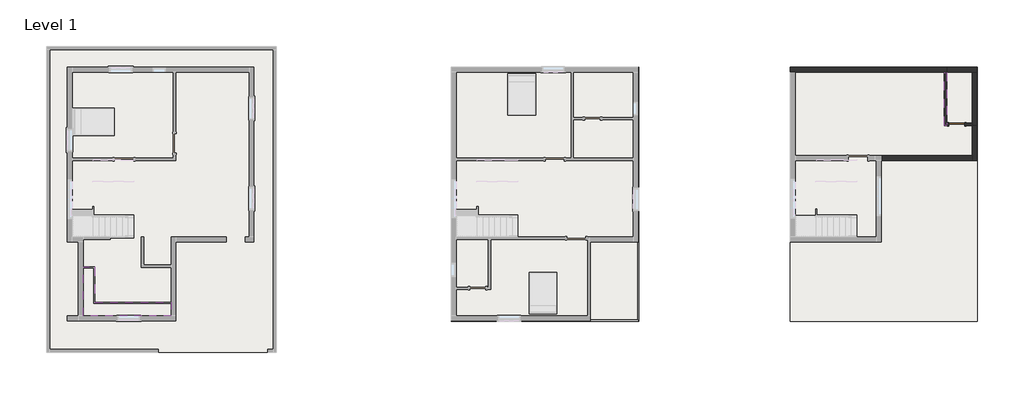
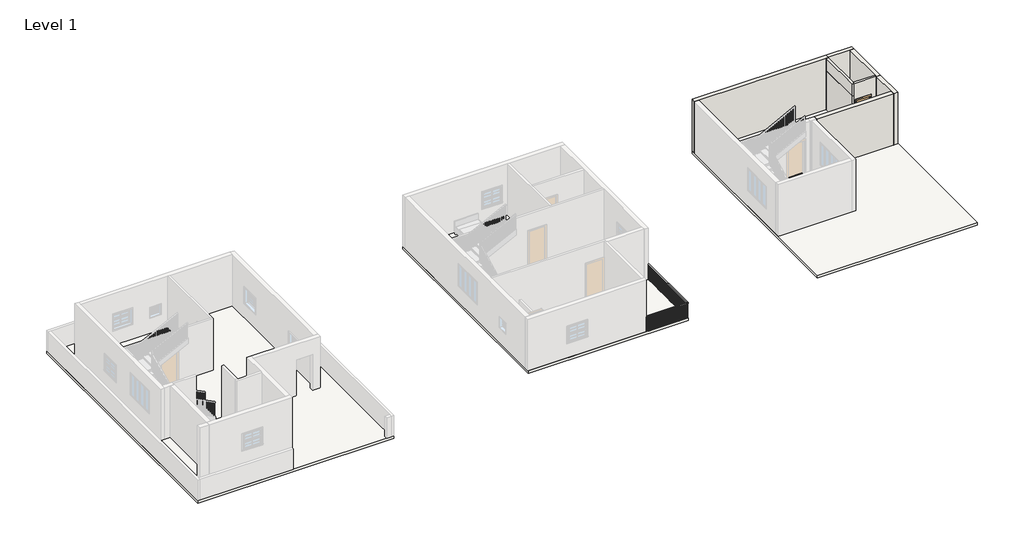
# One storey, part 2 of 8: 9 walls, 4 slabs, 1 door, 1 railing.
"""IFC4 building model written with IfcOpenShell, lengths in millimetres."""

from ifc_helpers import new_model, si_unit, frame, origin, origin_with_axes, place, context, project, spatial, polyline, outline, extrude, faceted_brep, transform, mapped, element, save
from components import door_f2b275c1

model = new_model("IFC4")

# Units and contexts
model_context = context("Model", 3, world=origin())
ifc_project = project(units=[si_unit("LENGTHUNIT", "METRE", prefix="MILLI")], contexts=[model_context])

# Site, building, storey
site = spatial("IfcSite", under=ifc_project)
building = spatial("IfcBuilding", under=site)
storey = spatial("IfcBuildingStorey", under=building, Name="Level 1", Elevation=0.0)

# Door
placement = place(None, origin())
door_shape = door_f2b275c1(model_context)
element("IfcDoor", 1, ObjectType="Single-Flush : door 2'6\"", at=placement, inside=storey, context=model_context, shape_type="MappedRepresentation", body=[
    mapped(door_shape, transform((19519.092447, 4272.7100713, 0.0), x_axis=(-1.0, 0.0, 0.0), y_axis=(0.0, -1.0, 0.0), z_axis=(0.0, 0.0, 1.0))),
])

# Railing
element("IfcRailing", 2, ObjectType="Handrail - Rectangular", at=placement, inside=storey, context=model_context, shape_type="SolidModel", body=[
    faceted_brep([(2026.2691518, -5093.5399287, 914.4), (2026.2691518, -5093.5399287, 863.6), (2026.2691518, -5144.3399287, 863.6), (2026.2691518, -5144.3399287, 914.4), (4286.8691518, -5093.5399287, 914.4), (4286.8691518, -5093.5399287, 863.6), (4337.6691518, -5144.3399287, 863.6), (4337.6691518, -5144.3399287, 914.4), (4286.8691518, -1347.0399287, 914.4), (4337.6691518, -1347.0399287, 914.4), (4337.6691518, -1347.0399287, 863.6), (4286.8691518, -1347.0399287, 863.6)], [[[0, 1, 2, 3]], [[1, 0, 4, 5]], [[2, 1, 5, 6]], [[3, 2, 6, 7]], [[0, 3, 7, 4]], [[8, 9, 10, 11]], [[5, 4, 8, 11]], [[6, 5, 11, 10]], [[7, 6, 10, 9]], [[4, 7, 9, 8]]]),
    extrude(outline(polyline([(4321.7941518, -1369.2649287), (4302.7441518, -1369.2649287), (4302.7441518, -1350.2149287), (4321.7941518, -1350.2149287), (4321.7941518, -1369.2649287)])), origin_with_axes(), (0.0, 0.0, 1.0), 863.6),
    extrude(outline(polyline([(4321.7941518, -1470.8649287), (4302.7441518, -1470.8649287), (4302.7441518, -1451.8149287), (4321.7941518, -1451.8149287), (4321.7941518, -1470.8649287)])), origin_with_axes(), (0.0, 0.0, 1.0), 863.6),
    extrude(outline(polyline([(4321.7941518, -1572.4649287), (4302.7441518, -1572.4649287), (4302.7441518, -1553.4149287), (4321.7941518, -1553.4149287), (4321.7941518, -1572.4649287)])), origin_with_axes(), (0.0, 0.0, 1.0), 863.6),
    extrude(outline(polyline([(4321.7941518, -1674.0649287), (4302.7441518, -1674.0649287), (4302.7441518, -1655.0149287), (4321.7941518, -1655.0149287), (4321.7941518, -1674.0649287)])), origin_with_axes(), (0.0, 0.0, 1.0), 863.6),
    extrude(outline(polyline([(4321.7941518, -1775.6649287), (4302.7441518, -1775.6649287), (4302.7441518, -1756.6149287), (4321.7941518, -1756.6149287), (4321.7941518, -1775.6649287)])), origin_with_axes(), (0.0, 0.0, 1.0), 863.6),
    extrude(outline(polyline([(4321.7941518, -1877.2649287), (4302.7441518, -1877.2649287), (4302.7441518, -1858.2149287), (4321.7941518, -1858.2149287), (4321.7941518, -1877.2649287)])), origin_with_axes(), (0.0, 0.0, 1.0), 863.6),
    extrude(outline(polyline([(4321.7941518, -1978.8649287), (4302.7441518, -1978.8649287), (4302.7441518, -1959.8149287), (4321.7941518, -1959.8149287), (4321.7941518, -1978.8649287)])), origin_with_axes(), (0.0, 0.0, 1.0), 863.6),
    extrude(outline(polyline([(4321.7941518, -2080.4649287), (4302.7441518, -2080.4649287), (4302.7441518, -2061.4149287), (4321.7941518, -2061.4149287), (4321.7941518, -2080.4649287)])), origin_with_axes(), (0.0, 0.0, 1.0), 863.6),
    extrude(outline(polyline([(4321.7941518, -2182.0649287), (4302.7441518, -2182.0649287), (4302.7441518, -2163.0149287), (4321.7941518, -2163.0149287), (4321.7941518, -2182.0649287)])), origin_with_axes(), (0.0, 0.0, 1.0), 863.6),
    extrude(outline(polyline([(4321.7941518, -2283.6649287), (4302.7441518, -2283.6649287), (4302.7441518, -2264.6149287), (4321.7941518, -2264.6149287), (4321.7941518, -2283.6649287)])), origin_with_axes(), (0.0, 0.0, 1.0), 863.6),
    extrude(outline(polyline([(4321.7941518, -2385.2649287), (4302.7441518, -2385.2649287), (4302.7441518, -2366.2149287), (4321.7941518, -2366.2149287), (4321.7941518, -2385.2649287)])), origin_with_axes(), (0.0, 0.0, 1.0), 863.6),
    extrude(outline(polyline([(4321.7941518, -2486.8649287), (4302.7441518, -2486.8649287), (4302.7441518, -2467.8149287), (4321.7941518, -2467.8149287), (4321.7941518, -2486.8649287)])), origin_with_axes(), (0.0, 0.0, 1.0), 863.6),
    extrude(outline(polyline([(4321.7941518, -2588.4649287), (4302.7441518, -2588.4649287), (4302.7441518, -2569.4149287), (4321.7941518, -2569.4149287), (4321.7941518, -2588.4649287)])), origin_with_axes(), (0.0, 0.0, 1.0), 863.6),
    extrude(outline(polyline([(4321.7941518, -2690.0649287), (4302.7441518, -2690.0649287), (4302.7441518, -2671.0149287), (4321.7941518, -2671.0149287), (4321.7941518, -2690.0649287)])), origin_with_axes(), (0.0, 0.0, 1.0), 863.6),
    extrude(outline(polyline([(4321.7941518, -2791.6649287), (4302.7441518, -2791.6649287), (4302.7441518, -2772.6149287), (4321.7941518, -2772.6149287), (4321.7941518, -2791.6649287)])), origin_with_axes(), (0.0, 0.0, 1.0), 863.6),
    extrude(outline(polyline([(4321.7941518, -2893.2649287), (4302.7441518, -2893.2649287), (4302.7441518, -2874.2149287), (4321.7941518, -2874.2149287), (4321.7941518, -2893.2649287)])), origin_with_axes(), (0.0, 0.0, 1.0), 863.6),
    extrude(outline(polyline([(4321.7941518, -2994.8649287), (4302.7441518, -2994.8649287), (4302.7441518, -2975.8149287), (4321.7941518, -2975.8149287), (4321.7941518, -2994.8649287)])), origin_with_axes(), (0.0, 0.0, 1.0), 863.6),
    extrude(outline(polyline([(4321.7941518, -3096.4649287), (4302.7441518, -3096.4649287), (4302.7441518, -3077.4149287), (4321.7941518, -3077.4149287), (4321.7941518, -3096.4649287)])), origin_with_axes(), (0.0, 0.0, 1.0), 863.6),
    extrude(outline(polyline([(4321.7941518, -3198.0649287), (4302.7441518, -3198.0649287), (4302.7441518, -3179.0149287), (4321.7941518, -3179.0149287), (4321.7941518, -3198.0649287)])), origin_with_axes(), (0.0, 0.0, 1.0), 863.6),
    extrude(outline(polyline([(4321.7941518, -3299.6649287), (4302.7441518, -3299.6649287), (4302.7441518, -3280.6149287), (4321.7941518, -3280.6149287), (4321.7941518, -3299.6649287)])), origin_with_axes(), (0.0, 0.0, 1.0), 863.6),
    extrude(outline(polyline([(4321.7941518, -3401.2649287), (4302.7441518, -3401.2649287), (4302.7441518, -3382.2149287), (4321.7941518, -3382.2149287), (4321.7941518, -3401.2649287)])), origin_with_axes(), (0.0, 0.0, 1.0), 863.6),
    extrude(outline(polyline([(4321.7941518, -3502.8649287), (4302.7441518, -3502.8649287), (4302.7441518, -3483.8149287), (4321.7941518, -3483.8149287), (4321.7941518, -3502.8649287)])), origin_with_axes(), (0.0, 0.0, 1.0), 863.6),
    extrude(outline(polyline([(4321.7941518, -3604.4649287), (4302.7441518, -3604.4649287), (4302.7441518, -3585.4149287), (4321.7941518, -3585.4149287), (4321.7941518, -3604.4649287)])), origin_with_axes(), (0.0, 0.0, 1.0), 863.6),
    extrude(outline(polyline([(4321.7941518, -3706.0649287), (4302.7441518, -3706.0649287), (4302.7441518, -3687.0149287), (4321.7941518, -3687.0149287), (4321.7941518, -3706.0649287)])), origin_with_axes(), (0.0, 0.0, 1.0), 863.6),
    extrude(outline(polyline([(4321.7941518, -3807.6649287), (4302.7441518, -3807.6649287), (4302.7441518, -3788.6149287), (4321.7941518, -3788.6149287), (4321.7941518, -3807.6649287)])), origin_with_axes(), (0.0, 0.0, 1.0), 863.6),
    extrude(outline(polyline([(4321.7941518, -3909.2649287), (4302.7441518, -3909.2649287), (4302.7441518, -3890.2149287), (4321.7941518, -3890.2149287), (4321.7941518, -3909.2649287)])), origin_with_axes(), (0.0, 0.0, 1.0), 863.6),
    extrude(outline(polyline([(4321.7941518, -4010.8649287), (4302.7441518, -4010.8649287), (4302.7441518, -3991.8149287), (4321.7941518, -3991.8149287), (4321.7941518, -4010.8649287)])), origin_with_axes(), (0.0, 0.0, 1.0), 863.6),
    extrude(outline(polyline([(4321.7941518, -4112.4649287), (4302.7441518, -4112.4649287), (4302.7441518, -4093.4149287), (4321.7941518, -4093.4149287), (4321.7941518, -4112.4649287)])), origin_with_axes(), (0.0, 0.0, 1.0), 863.6),
    extrude(outline(polyline([(4321.7941518, -4214.0649287), (4302.7441518, -4214.0649287), (4302.7441518, -4195.0149287), (4321.7941518, -4195.0149287), (4321.7941518, -4214.0649287)])), origin_with_axes(), (0.0, 0.0, 1.0), 863.6),
    extrude(outline(polyline([(4321.7941518, -4315.6649287), (4302.7441518, -4315.6649287), (4302.7441518, -4296.6149287), (4321.7941518, -4296.6149287), (4321.7941518, -4315.6649287)])), origin_with_axes(), (0.0, 0.0, 1.0), 863.6),
    extrude(outline(polyline([(4321.7941518, -4417.2649287), (4302.7441518, -4417.2649287), (4302.7441518, -4398.2149287), (4321.7941518, -4398.2149287), (4321.7941518, -4417.2649287)])), origin_with_axes(), (0.0, 0.0, 1.0), 863.6),
    extrude(outline(polyline([(4321.7941518, -4518.8649287), (4302.7441518, -4518.8649287), (4302.7441518, -4499.8149287), (4321.7941518, -4499.8149287), (4321.7941518, -4518.8649287)])), origin_with_axes(), (0.0, 0.0, 1.0), 863.6),
    extrude(outline(polyline([(4321.7941518, -4620.4649287), (4302.7441518, -4620.4649287), (4302.7441518, -4601.4149287), (4321.7941518, -4601.4149287), (4321.7941518, -4620.4649287)])), origin_with_axes(), (0.0, 0.0, 1.0), 863.6),
    extrude(outline(polyline([(4321.7941518, -4722.0649287), (4302.7441518, -4722.0649287), (4302.7441518, -4703.0149287), (4321.7941518, -4703.0149287), (4321.7941518, -4722.0649287)])), origin_with_axes(), (0.0, 0.0, 1.0), 863.6),
    extrude(outline(polyline([(4321.7941518, -4823.6649287), (4302.7441518, -4823.6649287), (4302.7441518, -4804.6149287), (4321.7941518, -4804.6149287), (4321.7941518, -4823.6649287)])), origin_with_axes(), (0.0, 0.0, 1.0), 863.6),
    extrude(outline(polyline([(4321.7941518, -4925.2649287), (4302.7441518, -4925.2649287), (4302.7441518, -4906.2149287), (4321.7941518, -4906.2149287), (4321.7941518, -4925.2649287)])), origin_with_axes(), (0.0, 0.0, 1.0), 863.6),
    extrude(outline(polyline([(4321.7941518, -5026.8649287), (4302.7441518, -5026.8649287), (4302.7441518, -5007.8149287), (4321.7941518, -5007.8149287), (4321.7941518, -5026.8649287)])), origin_with_axes(), (0.0, 0.0, 1.0), 863.6),
    extrude(outline(polyline([(4251.9441518, -5128.4649287), (4251.9441518, -5109.4149287), (4270.9941518, -5109.4149287), (4270.9941518, -5128.4649287), (4251.9441518, -5128.4649287)])), origin_with_axes(), (0.0, 0.0, 1.0), 863.6),
    extrude(outline(polyline([(4150.3441518, -5128.4649287), (4150.3441518, -5109.4149287), (4169.3941518, -5109.4149287), (4169.3941518, -5128.4649287), (4150.3441518, -5128.4649287)])), origin_with_axes(), (0.0, 0.0, 1.0), 863.6),
    extrude(outline(polyline([(4048.7441518, -5128.4649287), (4048.7441518, -5109.4149287), (4067.7941518, -5109.4149287), (4067.7941518, -5128.4649287), (4048.7441518, -5128.4649287)])), origin_with_axes(), (0.0, 0.0, 1.0), 863.6),
    extrude(outline(polyline([(3947.1441518, -5128.4649287), (3947.1441518, -5109.4149287), (3966.1941518, -5109.4149287), (3966.1941518, -5128.4649287), (3947.1441518, -5128.4649287)])), origin_with_axes(), (0.0, 0.0, 1.0), 863.6),
    extrude(outline(polyline([(3845.5441518, -5128.4649287), (3845.5441518, -5109.4149287), (3864.5941518, -5109.4149287), (3864.5941518, -5128.4649287), (3845.5441518, -5128.4649287)])), origin_with_axes(), (0.0, 0.0, 1.0), 863.6),
    extrude(outline(polyline([(3743.9441518, -5128.4649287), (3743.9441518, -5109.4149287), (3762.9941518, -5109.4149287), (3762.9941518, -5128.4649287), (3743.9441518, -5128.4649287)])), origin_with_axes(), (0.0, 0.0, 1.0), 863.6),
    extrude(outline(polyline([(3642.3441518, -5128.4649287), (3642.3441518, -5109.4149287), (3661.3941518, -5109.4149287), (3661.3941518, -5128.4649287), (3642.3441518, -5128.4649287)])), origin_with_axes(), (0.0, 0.0, 1.0), 863.6),
    extrude(outline(polyline([(3540.7441518, -5128.4649287), (3540.7441518, -5109.4149287), (3559.7941518, -5109.4149287), (3559.7941518, -5128.4649287), (3540.7441518, -5128.4649287)])), origin_with_axes(), (0.0, 0.0, 1.0), 863.6),
    extrude(outline(polyline([(3439.1441518, -5128.4649287), (3439.1441518, -5109.4149287), (3458.1941518, -5109.4149287), (3458.1941518, -5128.4649287), (3439.1441518, -5128.4649287)])), origin_with_axes(), (0.0, 0.0, 1.0), 863.6),
    extrude(outline(polyline([(3337.5441518, -5128.4649287), (3337.5441518, -5109.4149287), (3356.5941518, -5109.4149287), (3356.5941518, -5128.4649287), (3337.5441518, -5128.4649287)])), origin_with_axes(), (0.0, 0.0, 1.0), 863.6),
    extrude(outline(polyline([(3235.9441518, -5128.4649287), (3235.9441518, -5109.4149287), (3254.9941518, -5109.4149287), (3254.9941518, -5128.4649287), (3235.9441518, -5128.4649287)])), origin_with_axes(), (0.0, 0.0, 1.0), 863.6),
    extrude(outline(polyline([(3134.3441518, -5128.4649287), (3134.3441518, -5109.4149287), (3153.3941518, -5109.4149287), (3153.3941518, -5128.4649287), (3134.3441518, -5128.4649287)])), origin_with_axes(), (0.0, 0.0, 1.0), 863.6),
    extrude(outline(polyline([(3032.7441518, -5128.4649287), (3032.7441518, -5109.4149287), (3051.7941518, -5109.4149287), (3051.7941518, -5128.4649287), (3032.7441518, -5128.4649287)])), origin_with_axes(), (0.0, 0.0, 1.0), 863.6),
    extrude(outline(polyline([(2931.1441518, -5128.4649287), (2931.1441518, -5109.4149287), (2950.1941518, -5109.4149287), (2950.1941518, -5128.4649287), (2931.1441518, -5128.4649287)])), origin_with_axes(), (0.0, 0.0, 1.0), 863.6),
    extrude(outline(polyline([(2829.5441518, -5128.4649287), (2829.5441518, -5109.4149287), (2848.5941518, -5109.4149287), (2848.5941518, -5128.4649287), (2829.5441518, -5128.4649287)])), origin_with_axes(), (0.0, 0.0, 1.0), 863.6),
    extrude(outline(polyline([(2727.9441518, -5128.4649287), (2727.9441518, -5109.4149287), (2746.9941518, -5109.4149287), (2746.9941518, -5128.4649287), (2727.9441518, -5128.4649287)])), origin_with_axes(), (0.0, 0.0, 1.0), 863.6),
    extrude(outline(polyline([(2626.3441518, -5128.4649287), (2626.3441518, -5109.4149287), (2645.3941518, -5109.4149287), (2645.3941518, -5128.4649287), (2626.3441518, -5128.4649287)])), origin_with_axes(), (0.0, 0.0, 1.0), 863.6),
    extrude(outline(polyline([(2524.7441518, -5128.4649287), (2524.7441518, -5109.4149287), (2543.7941518, -5109.4149287), (2543.7941518, -5128.4649287), (2524.7441518, -5128.4649287)])), origin_with_axes(), (0.0, 0.0, 1.0), 863.6),
    extrude(outline(polyline([(2423.1441518, -5128.4649287), (2423.1441518, -5109.4149287), (2442.1941518, -5109.4149287), (2442.1941518, -5128.4649287), (2423.1441518, -5128.4649287)])), origin_with_axes(), (0.0, 0.0, 1.0), 863.6),
    extrude(outline(polyline([(2321.5441518, -5128.4649287), (2321.5441518, -5109.4149287), (2340.5941518, -5109.4149287), (2340.5941518, -5128.4649287), (2321.5441518, -5128.4649287)])), origin_with_axes(), (0.0, 0.0, 1.0), 863.6),
    extrude(outline(polyline([(2219.9441518, -5128.4649287), (2219.9441518, -5109.4149287), (2238.9941518, -5109.4149287), (2238.9941518, -5128.4649287), (2219.9441518, -5128.4649287)])), origin_with_axes(), (0.0, 0.0, 1.0), 863.6),
    extrude(outline(polyline([(2118.3441518, -5128.4649287), (2118.3441518, -5109.4149287), (2137.3941518, -5109.4149287), (2137.3941518, -5128.4649287), (2118.3441518, -5128.4649287)])), origin_with_axes(), (0.0, 0.0, 1.0), 863.6),
    extrude(outline(polyline([(4302.7441518, -5128.4649287), (4302.7441518, -5109.4149287), (4321.7941518, -5109.4149287), (4321.7941518, -5128.4649287), (4302.7441518, -5128.4649287)])), origin_with_axes(), (0.0, 0.0, 1.0), 863.6),
    extrude(outline(polyline([(4321.7941518, -1366.0899287), (4302.7441518, -1366.0899287), (4302.7441518, -1347.0399287), (4321.7941518, -1347.0399287), (4321.7941518, -1366.0899287)])), origin_with_axes(), (0.0, 0.0, 1.0), 863.6),
    extrude(outline(polyline([(2026.2691518, -5128.4649287), (2026.2691518, -5109.4149287), (2045.3191518, -5109.4149287), (2045.3191518, -5128.4649287), (2026.2691518, -5128.4649287)])), origin_with_axes(), (0.0, 0.0, 1.0), 863.6),
])

# Slabs
element("IfcSlab", 3, ObjectType="FLOOR 2\"", at=placement, inside=storey, context=model_context, shape_type="SweptSolid", body=[
    extrude(outline(polyline([(-21624.0789184, -2540.8399287), (-21624.0789184, -4255.3399287), (-17991.8789184, -4255.3399287), (-17991.8789184, -4890.3399287), (-22182.8789184, -4890.3399287), (-22182.8789184, -2540.8399287), (-21624.0789184, -2540.8399287)])), frame((0.0, 0.0, 1473.2), z_axis=(0.0, 0.0, 1.0), x_axis=(1.0, 0.0, 0.0)), (0.0, 0.0, 1.0), 50.8),
])
element("IfcSlab", 4, ObjectType="floor 6\"", at=placement, inside=storey, context=model_context, shape_type="SweptSolid", body=[
    extrude(outline(polyline([(-12962.6789184, 7987.4600713), (-12962.6789184, -6642.9399287), (-23935.4789184, -6642.9399287), (-23935.4789184, 7987.4600713), (-12962.6789184, 7987.4600713)])), frame((0.0, 0.0, -152.4), z_axis=(0.0, 0.0, 1.0), x_axis=(1.0, 0.0, 0.0)), (0.0, 0.0, 1.0), 152.4),
])
element("IfcSlab", 5, ObjectType="floor 6\"", at=placement, inside=storey, context=model_context, shape_type="SweptSolid", body=[
    extrude(outline(polyline([(4337.6691518, 6996.8600713), (4337.6691518, -5144.3399287), (-4603.1308482, -5144.3399287), (-4603.1308482, 6996.8600713), (4337.6691518, 6996.8600713)])), frame((0.0, 0.0, -152.4), z_axis=(0.0, 0.0, 1.0), x_axis=(1.0, 0.0, 0.0)), (0.0, 0.0, 1.0), 152.4),
])
element("IfcSlab", 6, ObjectType="floor 6\"", at=placement, inside=storey, context=model_context, shape_type="SweptSolid", body=[
    extrude(outline(polyline([(20516.042447, 6996.8600713), (20516.042447, -5144.3399287), (11575.242447, -5144.3399287), (11575.242447, 6996.8600713), (20516.042447, 6996.8600713)])), frame((0.0, 0.0, -152.4), z_axis=(0.0, 0.0, 1.0), x_axis=(1.0, 0.0, 0.0)), (0.0, 0.0, 1.0), 152.4),
])

# Walls
element("IfcWall", 7, ObjectType="WALL 4.5\"", at=placement, inside=storey, context=model_context, shape_type="Brep", body=[
    faceted_brep([(18928.542447, 6768.2600713, 0.0), (18928.542447, 6730.1600713, 0.0), (18928.542447, 6730.1600713, 2336.8), (18928.542447, 6730.1600713, 3048.0), (18928.542447, 6768.2600713, 3048.0), (19042.842447, 6768.2600713, 0.0), (19042.842447, 6768.2600713, 3048.0), (19042.842447, 6730.1600713, 3048.0), (19042.842447, 6730.1600713, 2336.8), (19042.842447, 6730.1600713, 0.0)], [[[0, 1, 2, 3, 4]], [[5, 6, 7, 8, 9]], [[1, 0, 5, 9]], [[4, 3, 7, 6]], [[0, 4, 6, 5]], [[1, 9, 8, 7, 3, 2]]]),
])
element("IfcWall", 8, ObjectType="WALL 4.5\"", at=placement, inside=storey, context=model_context, shape_type="Brep", body=[
    faceted_brep([(20262.042447, 4215.5600713, 3048.0), (19042.842447, 4215.5600713, 3048.0), (19042.842447, 4215.5600713, 2336.8), (19042.842447, 4215.5600713, 0.0), (19138.092447, 4215.5600713, 0.0), (19138.092447, 4215.5600713, 2032.0), (19900.092447, 4215.5600713, 2032.0), (19900.092447, 4215.5600713, 0.0), (20262.042447, 4215.5600713, 0.0), (19042.842447, 4329.8600713, 3048.0), (20262.042447, 4329.8600713, 3048.0), (20262.042447, 4329.8600713, 0.0), (19900.092447, 4329.8600713, 0.0), (19900.092447, 4329.8600713, 2032.0), (19138.092447, 4329.8600713, 2032.0), (19138.092447, 4329.8600713, 0.0), (19042.842447, 4329.8600713, 0.0)], [[[0, 1, 2, 3, 4, 5, 6, 7, 8]], [[9, 10, 11, 12, 13, 14, 15, 16]], [[3, 16, 15, 4]], [[11, 8, 7, 12]], [[1, 0, 10, 9]], [[0, 8, 11, 10]], [[14, 5, 4, 15]], [[6, 13, 12, 7]], [[13, 6, 5, 14]], [[1, 9, 16, 3, 2]]]),
])
element("IfcWall", 9, ObjectType="WALL 4.5\"", at=placement, inside=storey, context=model_context, shape_type="Brep", body=[
    faceted_brep([(18928.542447, 6730.1600713, 0.0), (18928.542447, 4215.5600713, 0.0), (18928.542447, 4215.5600713, 2336.8), (18928.542447, 6730.1600713, 2336.8), (19042.842447, 6730.1600713, 0.0), (19042.842447, 6730.1600713, 2336.8), (19042.842447, 4215.5600713, 2336.8), (19042.842447, 4215.5600713, 0.0), (19042.842447, 4329.8600713, 0.0)], [[[0, 1, 2, 3]], [[4, 5, 6, 7, 8]], [[1, 0, 4, 8, 7]], [[3, 2, 6, 5]], [[0, 3, 5, 4]], [[2, 1, 7, 6]]]),
])
element("IfcWall", 10, ObjectType="WALL 4.5\"", at=placement, inside=storey, context=model_context, shape_type="Brep", body=[
    faceted_brep([(18928.542447, 6730.1600713, 2336.8), (18928.542447, 4215.5600713, 2336.8), (18928.542447, 4215.5600713, 3048.0), (18928.542447, 6730.1600713, 3048.0), (19042.842447, 6730.1600713, 2336.8), (19042.842447, 6730.1600713, 3048.0), (19042.842447, 4329.8600713, 3048.0), (19042.842447, 4215.5600713, 3048.0), (19042.842447, 4215.5600713, 2336.8)], [[[0, 1, 2, 3]], [[4, 5, 6, 7, 8]], [[1, 0, 4, 8]], [[3, 2, 7, 6, 5]], [[0, 3, 5, 4]], [[2, 1, 8, 7]]]),
])
element("IfcWall", 11, ObjectType="WALL 9\"", at=placement, inside=storey, context=model_context, shape_type="Brep", body=[
    faceted_brep([(11575.242447, 6768.2600713, 0.0), (11803.842447, 6768.2600713, 0.0), (18928.542447, 6768.2600713, 0.0), (19042.842447, 6768.2600713, 0.0), (19055.542447, 6768.2600713, 0.0), (19055.542447, 6768.2600713, 3048.0), (19042.842447, 6768.2600713, 3048.0), (18928.542447, 6768.2600713, 3048.0), (11803.842447, 6768.2600713, 3048.0), (11575.242447, 6768.2600713, 3048.0), (11575.242447, 6996.8600713, 0.0), (11575.242447, 6996.8600713, 3048.0), (19055.542447, 6996.8600713, 3048.0), (19055.542447, 6996.8600713, 0.0)], [[[0, 1, 2, 3, 4, 5, 6, 7, 8, 9]], [[10, 11, 12, 13]], [[4, 3, 2, 1, 0, 10, 13]], [[5, 4, 13, 12]], [[0, 9, 11, 10]], [[9, 8, 7, 6, 5, 12, 11]]]),
])
element("IfcWall", 12, ObjectType="WALL 9\"", at=placement, inside=storey, context=model_context, shape_type="Brep", body=[
    faceted_brep([(20262.042447, 6768.2600713, 0.0), (20262.042447, 4329.8600713, 0.0), (20262.042447, 4215.5600713, 0.0), (20262.042447, 4202.8600713, 0.0), (20262.042447, 4202.8600713, 3048.0), (20262.042447, 4215.5600713, 3048.0), (20262.042447, 4329.8600713, 3048.0), (20262.042447, 6768.2600713, 3048.0), (20490.642447, 6768.2600713, 0.0), (20490.642447, 6768.2600713, 3048.0), (20490.642447, 4202.8600713, 3048.0), (20490.642447, 4202.8600713, 0.0)], [[[0, 1, 2, 3, 4, 5, 6, 7]], [[8, 9, 10, 11]], [[3, 2, 1, 0, 8, 11]], [[4, 3, 11, 10]], [[0, 7, 9, 8]], [[7, 6, 5, 4, 10, 9]]]),
])
element("IfcWall", 13, ObjectType="WALL 9\"", at=placement, inside=storey, context=model_context, shape_type="SweptSolid", body=[
    extrude(outline(polyline([(15956.742447, 2767.7600713), (20262.042447, 2767.7600713), (20262.042447, 2539.1600713), (15956.742447, 2539.1600713), (15956.742447, 2767.7600713)])), origin_with_axes(), (0.0, 0.0, 1.0), 3048.0),
])
element("IfcWall", 14, ObjectType="WALL 9\"", at=placement, inside=storey, context=model_context, shape_type="Brep", body=[
    faceted_brep([(19055.542447, 6768.2600713, 0.0), (20262.042447, 6768.2600713, 0.0), (20490.642447, 6768.2600713, 0.0), (20490.642447, 6768.2600713, 3048.0), (20262.042447, 6768.2600713, 3048.0), (19055.542447, 6768.2600713, 3048.0), (19055.542447, 6996.8600713, 0.0), (19055.542447, 6996.8600713, 3048.0), (20490.642447, 6996.8600713, 3048.0), (20490.642447, 6996.8600713, 0.0)], [[[0, 1, 2, 3, 4, 5]], [[6, 7, 8, 9]], [[2, 1, 0, 6, 9]], [[0, 5, 7, 6]], [[3, 2, 9, 8]], [[5, 4, 3, 8, 7]]]),
])
element("IfcWall", 15, ObjectType="WALL 9\"", at=placement, inside=storey, context=model_context, shape_type="Brep", body=[
    faceted_brep([(20262.042447, 4202.8600713, 0.0), (20262.042447, 2767.7600713, 0.0), (20262.042447, 2539.1600713, 0.0), (20262.042447, 2539.1600713, 3048.0), (20262.042447, 2767.7600713, 3048.0), (20262.042447, 4202.8600713, 3048.0), (20490.642447, 4202.8600713, 0.0), (20490.642447, 4202.8600713, 3048.0), (20490.642447, 2539.1600713, 3048.0), (20490.642447, 2539.1600713, 0.0)], [[[0, 1, 2, 3, 4, 5]], [[6, 7, 8, 9]], [[2, 1, 0, 6, 9]], [[0, 5, 7, 6]], [[3, 2, 9, 8]], [[5, 4, 3, 8, 7]]]),
])

save(model, "model.ifc")

# Revit data of these elements
# Type "Single-Flush : door 2'6\""
#   Type Mark = "10"
#   Construction Type Id = "MDOOR"
#   Assembly Code = "C1020"
#   Analytic Construction = "Metal"
#   Thickness = 0' - 2"
#   Heat Transfer Coefficient (U) = 0.651978 BTU/(h·ft²·°F)
#   Height = 6' - 8"
#   Trim Projection Ext = 0' - 1"
#   Trim Projection Int = 0' - 1"
#   Trim Width = 0' - 3"
#   Width = 2' - 6"
#   Define Thermal Properties by = 1
#   Door Material = Door - Panel
#   Frame Material = Door - Frame
#   Visual Light Transmittance = 0
#   Solar Heat Gain Coefficient = 0
#   Function = (empty or 0)
#   Wall Closure = (empty or 0)
# Type "Handrail - Rectangular"
#   Assembly Code = "C2010400"
#   built-in parameter 1008612 = 0.0416667 (stored number, unit not read)
#   built-in parameter 1008611 = 0.0416667 (stored number, unit not read)
#   built-in parameter 1008609 = 0.333333 (stored number, unit not read)
#   built-in parameter 1008604 = 0.166667 (stored number, unit not read)
#   built-in parameter 1008603 = 0.166667 (stored number, unit not read)
#   Railing Height = 3' - 0"
#   built-in parameter 1008630 = 2
#   built-in parameter 1008610 = 2
#   built-in parameter 1008618 = Baluster - Square : 3/4"
# Type "FLOOR 2\""
#   Assembly Code = "B1010"
#   Function = 0
#   Layers, outside or top first: 0' - 2" no material (function 1)
# Type "floor 6\""
#   Assembly Code = "B1010"
#   Function = 0
#   Layers, outside or top first: 0' - 6" no material (function 1)
# Type "WALL 4.5\""
#   Assembly Code = "B2010"
#   Layers, outside or top first: 0' - 4 1/2" no material (function 1)
# Type "WALL 9\""
#   Assembly Code = "B2010"
#   Layers, outside or top first: 0' - 9" no material (function 1)
# Element 1 (IfcDoor, "Single-Flush : door 2'6\"")
#   Phase Created = New Construction
#   Materials on its faces: "Door - Frame", "Door - Panel"
# Element 2 (IfcRailing, "Handrail - Rectangular")
#   Phase Created = New Construction
# Element 3 (IfcSlab, "FLOOR 2\"")
#   Height Offset From Level = 5' - 0"
#   Phase Created = New Construction
#   Materials on its faces: "Default Floor", "TILES"
# Element 4 (IfcSlab, "floor 6\"")
#   Height Offset From Level = 0' - 0"
#   Phase Created = New Construction
#   Materials on its faces: "light shade", "Default Floor", "FLOOR T"
# Element 5 (IfcSlab, "floor 6\"")
#   Height Offset From Level = 0' - 0"
#   Phase Created = New Construction
#   Materials on its faces: "light shade", "Default Floor", "F WHITE"
# Element 6 (IfcSlab, "floor 6\"")
#   Height Offset From Level = 0' - 0"
#   Phase Created = New Construction
#   Materials on its faces: "light shade", "Default Floor", "MULTI F"
# Elements 7, 8 (IfcWall, "WALL 4.5\"")
#   Top Offset = 0' - 0"
#   Base Offset = 0' - 0"
#   Unconnected Height = 10' - 0"
#   wall height = 10' - 0"
#   Phase Created = New Construction
#   Base Constraint = Level 1
#   Materials on its faces: "Default Wall", "1 wall", "diff"
# Element 9 (IfcWall, "WALL 4.5\"")
#   Top Offset = 0' - 0"
#   Base Offset = 0' - 0"
#   Unconnected Height = 7' - 8"
#   wall height = 7' - 8"
#   Phase Created = New Construction
#   Base Constraint = Level 1
#   Materials on its faces: "Default Wall", "1 wall", "diff"
# Element 10 (IfcWall, "WALL 4.5\"")
#   built-in parameter 1001111 = 7' - 8"
#   Top Offset = 0' - 0"
#   Base Offset = 7' - 8"
#   Unconnected Height = 2' - 4"
#   wall height = 2' - 4"
#   Phase Created = New Construction
#   Base Constraint = Level 1
#   Materials on its faces: "Default Wall", "1 wall", "diff"
# Elements 11, 13, 15 (IfcWall, "WALL 9\"")
#   Top Offset = 0' - 0"
#   Base Offset = 0' - 0"
#   Unconnected Height = 10' - 0"
#   wall height = 10' - 0"
#   Phase Created = New Construction
#   Base Constraint = Level 1
#   Materials on its faces: "Default Wall", "1 wall"
# Elements 12, 14 (IfcWall, "WALL 9\"")
#   Top Offset = 0' - 0"
#   Base Offset = 0' - 0"
#   Unconnected Height = 10' - 0"
#   wall height = 10' - 0"
#   Phase Created = New Construction
#   Base Constraint = Level 1
#   Materials on its faces: "Default Wall", "diff"
# Materials
#   "Door - Panel": class "Wood", colour RGB 210 159 95, transparency 0, Cost = 0
#   "Door - Frame": colour RGB 118 70 51, transparency 0, Cost = 0
#   "Default Floor": colour RGB 128 128 128, transparency 0, Cost = 0
#   "TILES": class "Generic", colour RGB 120 120 120, transparency 0, Cost = 0
#   "light shade": class "Generic", colour RGB 120 120 120, transparency 0, Cost = 0
#   "FLOOR T": class "Generic", colour RGB 120 120 120, transparency 0, Cost = 0
#   "F WHITE": class "Generic", colour RGB 120 120 120, transparency 0, Cost = 0
#   "MULTI F": class "Generic", colour RGB 120 120 120, transparency 0, Cost = 0
#   "Default Wall": colour RGB 128 128 128, transparency 0, Cost = 0
#   "1 wall": class "Glass", colour RGB 0 0 255, transparency 0.75, Cost = 0
#   "diff": class "Generic", colour RGB 120 120 120, transparency 0, Cost = 0
